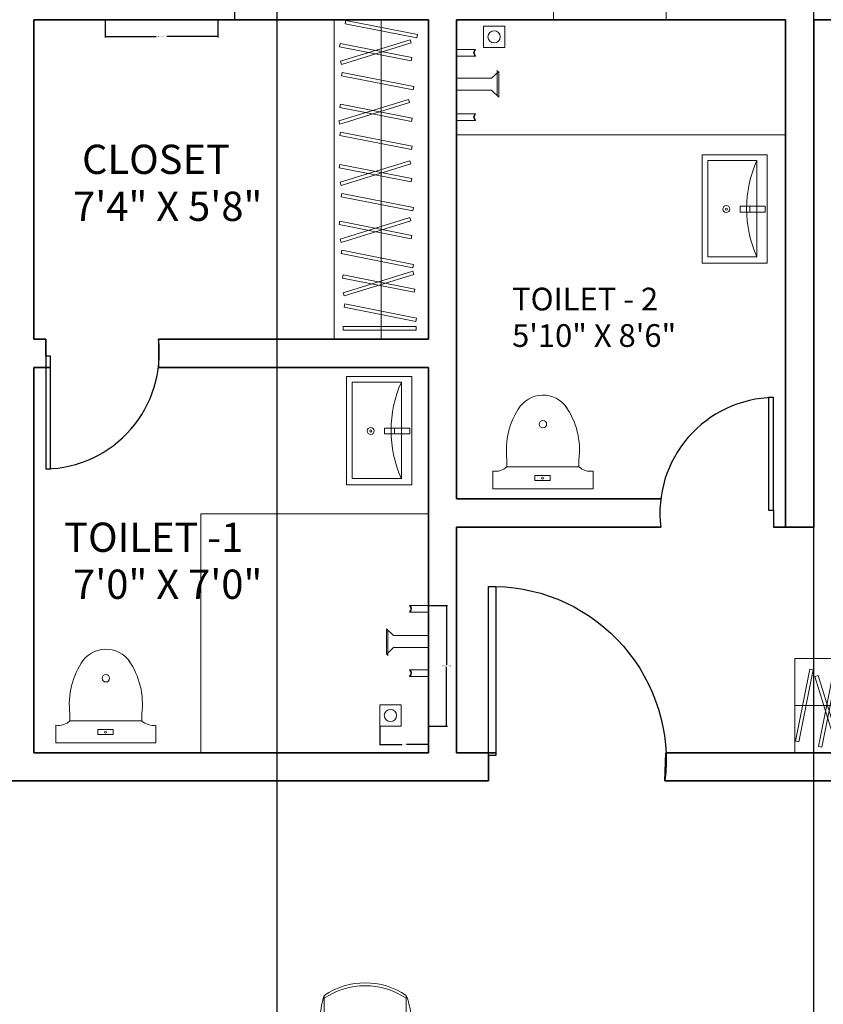
# Model space of a CAD drawing. Units: inches. Extents: x -61 to 1599, y -1316 to 257.
# Tile 202 of 204: x 1213 to 1384, y -61 to 149. Entities that reach past the tile are written whole.
import ezdxf

# ---------------------------------------------------------------- set-up
doc = ezdxf.new("R2010")
doc.units = ezdxf.units.IN
doc.header["$MEASUREMENT"] = 0
doc.linetypes.add('ACAD_ISO02W100', pattern=[15, 12, -3])
for name, color, linetype, lineweight in [('A-ANNO-DIMS', 2, 'Continuous', 18), ('A-AREA-IDEN', 1, 'Continuous', 18), ('A-FLOR-CASE', 8, 'Continuous', 18), ('A-FLOR-FIXT', 8, 'Continuous', 18), ('A-WALL-JAMB', 4, 'ACAD_ISO02W100', 25), ('DOORS', 2, 'Continuous', 25), ('FURNITURE', 83, 'Continuous', 18), ('WALLS', 4, 'Continuous', 35), ('WINDOWS', 220, 'Continuous', 18)]:
    doc.layers.add(name, color=color, linetype=linetype, lineweight=lineweight)
doc.styles.get("Standard").update_dxf_attribs({"font": 'arial.ttf'})
doc.dimstyles.get("Standard").update_dxf_attribs({"dimtxt": 0.18, "dimasz": 0.18, "dimexe": 0.18, "dimexo": 0.0625, "dimgap": 0.09, "dimtad": 0, "dimtih": 1, "dimtoh": 1, "dimdec": 0, "dimzin": 0, "dimdsep": 46, "dimlunit": 3, "dimtxsty": 'Standard', "dimcen": 0.09, "dimadec": 0, "dimazin": 0, "dimtfac": 1, "dimtdec": 0, "dimtofl": 0, "dimtmove": 0, "dimatfit": 3, "dimfxl": 1, "dimtolj": 1, "dimtzin": 0, "dimarcsym": 0})

# ---------------------------------------------------------------- blocks, each defined once
blk = doc.blocks.new('DOOR-SWING-24')
blk.add_line((0, 0), (0, 3.6))
blk.add_lwpolyline([(0, 0), (0, -24), (1.05, -24), (1.05, 0)], close=True)
blk.add_arc((-0.44, 0.62), 24.62, 271.0259, 6.9559)
blk = doc.blocks.new('DOOR-SWING-36')
blk.add_line((0, 0), (0, -5.4))
blk.add_lwpolyline([(0, 0), (0, 36), (-1.57, 36), (-1.57, 0)], close=True)
blk.add_arc((-0.74, -1.08), 37.09, 91.2913, 186.6905)
blk = doc.blocks.new('WIN-24IN')
for p, q in [((0, 4.5), (0, 9)), ((0, 9), (0, 0)), ((24, 9), (24, 0)), ((0, 5.19), (24, 5.19)), ((0, 4.5), (24, 4.5))]:
    blk.add_line(p, q)
blk = doc.blocks.new('WC-FLOOR-MOUNT')
for p, q in [((3.02, 4.69), (3.02, 6.17)), ((3.02, 4.69), (18.31, 4.69)), ((18.31, 4.69), (18.31, 6.17)), ((0, 0), (0, 3.75)), ((21.33, 0), (21.33, 3.75)), ((0, 0), (21.33, 0))]:
    blk.add_line(p, q)
blk.add_lwpolyline([(12.24, 1.73), (8.96, 1.73), (8.96, 2.81), (12.24, 2.81)], close=True)
for centre, radius in [((10.67, 13.73), 0.792), ((10.6, 2.27), 0.208)]:
    blk.add_circle(centre, radius)
for centre, radius, start, end in [((10.67, 13.73), 6.18, 27.6844, 141.4697), ((19.05, 8.26), 16.17, 144.824, 187.4232), ((2.28, 8.26), 16.17, 352.5768, 35.176), ((0.56, 7.25), 3.55, 260.8586, 313.6993), ((20.77, 7.25), 3.55, 226.3007, 279.1414)]:
    blk.add_arc(centre, radius, start, end)
blk = doc.blocks.new('LAVATORY-WALL')
blk.add_line((10.19, 12.11), (10.19, 10.88))
for points in [[(13.87, 0), (0, 0), (0, 23.07), (13.87, 23.07)], [(13.87, 0), (0, 0), (0, 23.07), (13.87, 23.07)], [(1.2, 1.34), (1.2, 21.88), (11.67, 21.88), (11.67, 1.34)], [(8.09, 10.88), (8.09, 12.11), (13.47, 12.11), (13.47, 10.88)]]:
    blk.add_lwpolyline(points, close=True)
for radius in [0.74, 0.233]:
    blk.add_circle((5.16, 11.5), radius)
blk.add_arc((34.73, 11.61), 25.25, 155.9939, 204.0061)
blk = doc.blocks.new('SHOWER-FITTINGS')
for p, q in [((10.35, 25.72), (6.31, 25.72)), ((10.35, 24.3), (6.31, 24.3)), ((10.35, 23), (10.35, 23)), ((2.92, 19.29), (1.4, 20.76)), ((1.4, 15.27), (1.4, 20.76)), ((1.69, 14.98), (1.69, 20.48)), ((10.35, 19.29), (2.92, 19.29)), ((2.92, 16.74), (1.4, 15.27)), ((10.35, 16.74), (2.92, 16.74)), ((10.35, 12.03), (6.31, 12.03)), ((10.35, 10.61), (6.31, 10.61))]:
    blk.add_line(p, q)
blk.add_lwpolyline([(4.52, 0), (0, 0), (0, 4.57), (4.52, 4.57)], close=True)
blk.add_circle((2.26, 2.29), 1.31)
for points in [[(6.31, 24.3), (6.45, 24.53), (6.75, 25), (6.46, 25.48), (6.31, 25.72)], [(6.45, 24.3), (6.59, 24.53), (6.88, 25), (6.59, 25.48), (6.45, 25.72)], [(6.31, 10.61), (6.45, 10.84), (6.75, 11.31), (6.46, 11.78), (6.31, 12.03)], [(6.45, 10.61), (6.59, 10.84), (6.88, 11.31), (6.59, 11.78), (6.45, 12.03)]]:
    blk.add_open_spline(points, degree=3, knots=[0, 0, 0, 0, 0.7501, 1.532449, 1.532449, 1.532449, 1.532449])
blk = doc.blocks.new('SHOWER-FITTINGS-2')
for p, q in [((0, 15.11), (4.04, 15.11)), ((0, 13.69), (4.04, 13.69)), ((8.66, 10.73), (8.66, 5.24)), ((0, 8.98), (7.43, 8.98)), ((7.43, 8.98), (8.95, 10.45)), ((8.95, 10.45), (8.95, 4.96)), ((0, 6.43), (7.43, 6.43)), ((7.43, 6.43), (8.95, 4.96)), ((0, 1.42), (4.04, 1.42)), ((0, 0), (4.04, 0))]:
    blk.add_line(p, q)
blk.add_lwpolyline([(10.23, 15.5), (5.71, 15.5), (5.71, 20.08), (10.23, 20.08)], close=True)
blk.add_circle((7.97, 17.79), 1.31)
for points in [[(3.91, 15.11), (3.76, 14.88), (3.47, 14.41), (3.76, 13.94), (3.91, 13.69)], [(4.04, 15.11), (3.9, 14.88), (3.6, 14.41), (3.89, 13.94), (4.04, 13.69)], [(3.91, 1.42), (3.76, 1.19), (3.47, 0.72), (3.76, 0.24), (3.91, 0)], [(4.04, 1.42), (3.9, 1.19), (3.6, 0.72), (3.89, 0.24), (4.04, 0)]]:
    blk.add_open_spline(points, degree=3, knots=[0, 0, 0, 0, 0.7501, 1.532449, 1.532449, 1.532449, 1.532449])
blk = doc.blocks.new('DINING-CHAIR')
for p, q in [((0.9, 2.16), (0.9, 13.35)), ((18.35, 2.16), (18.35, 13.35))]:
    blk.add_line(p, q)
for centre, radius, start, end in [((9.63, 0.52), 15.52, 55.8098, 124.1902), ((9.63, -0.1), 15.52, 55.8098, 124.1902), ((17.78, 7.76), 17.78, 161.6455, 198.3545), ((4.51, 7.76), 14.92, 337.9646, 22.0354), ((9.63, 12.87), 12.87, 227.332, 312.668)]:
    blk.add_arc(centre, radius, start, end)
blk = doc.blocks.new('WARDROBE-HANGING')
blk.add_line((10.05, 0), (10.05, 68))
for points in [[(20.09, 0), (0, 0), (0, 68), (20.09, 68)], [(2.48, 67.85), (17.75, 64.85), (17.61, 64.14), (2.34, 67.15)], [(1.32, 62.96), (16.59, 59.95), (16.45, 59.25), (1.19, 62.25)], [(1.35, 59.16), (16.22, 63.73), (16.43, 63.04), (1.56, 58.47)], [(1.71, 56.78), (16.98, 53.78), (16.84, 53.07), (1.57, 56.08)], [(1, 46.47), (15.87, 51.04), (16.08, 50.35), (1.21, 45.78)], [(1.39, 50.01), (16.66, 47.01), (16.52, 46.3), (1.26, 49.31)], [(1.36, 44.09), (16.63, 41.09), (16.49, 40.38), (1.23, 43.38)], [(1.28, 33.41), (16.16, 37.98), (16.37, 37.29), (1.49, 32.72)], [(1.26, 37.2), (16.53, 34.2), (16.39, 33.49), (1.12, 36.5)], [(1.65, 31.03), (16.92, 28.03), (16.78, 27.32), (1.51, 30.32)], [(1.28, 21.3), (16.15, 25.87), (16.36, 25.18), (1.49, 20.61)], [(1.26, 25.09), (16.53, 22.09), (16.39, 21.38), (1.12, 24.39)], [(1.65, 18.92), (16.91, 15.92), (16.78, 15.21), (1.51, 18.21)], [(1.91, 13.69), (17.17, 10.68), (17.04, 9.98), (1.77, 12.98)], [(1.93, 9.89), (16.8, 14.46), (17.01, 13.77), (2.14, 9.2)], [(2.29, 7.51), (17.56, 4.51), (17.42, 3.8), (2.16, 6.81)], [(17.49, 1.96), (1.93, 1.96), (1.93, 2.68), (17.49, 2.68)]]:
    blk.add_lwpolyline(points, close=True)
blk = doc.blocks.new('*D614')
at = {"layer": 'A-ANNO-DIMS', "color": 0, "lineweight": -2, "transparency": 16777216}
for p, q in [((1230.88, 148.61), (1230.88, 144.9)), ((1254.88, 148.61), (1254.88, 144.9)), ((1231.06, 145.08), (1241.76, 145.08)), ((1254.7, 145.08), (1244, 145.08))]:
    blk.add_line(p, q, dxfattribs=at)
at = {"layer": 'A-ANNO-DIMS', "color": 0, "transparency": 16777216}
for points in [[(1231.06, 145.11), (1231.06, 145.05), (1230.88, 145.08)], [(1254.7, 145.11), (1254.7, 145.05), (1254.88, 145.08)]]:
    blk.add_solid(points, dxfattribs=at)
at = {"layer": 'DEFPOINTS', "color": 0, "transparency": 16777216}
for p in [(1230.88, 148.68), (1254.88, 148.68), (1254.88, 145.08)]:
    blk.add_point(p, dxfattribs=at)
at = {"layer": 'A-ANNO-DIMS', "color": 0, "transparency": 16777216, "insert": (1242.88, 145.08), "char_height": 0.18, "attachment_point": 5}
blk.add_mtext('\\A1;WINDOW 24 TYP.', dxfattribs=at)
blk = doc.blocks.new('*D615')
at = {"layer": 'A-ANNO-DIMS', "color": 0, "lineweight": -2, "transparency": 16777216}
for p, q in [((1254.94, 157.68), (1258.66, 157.68)), ((1258.48, 157.5), (1258.48, 153.36)), ((1258.48, 148.86), (1258.48, 153)), ((1254.94, 148.68), (1258.66, 148.68))]:
    blk.add_line(p, q, dxfattribs=at)
at = {"layer": 'A-ANNO-DIMS', "color": 0, "transparency": 16777216}
for points in [[(1258.45, 157.5), (1258.51, 157.5), (1258.48, 157.68)], [(1258.45, 148.86), (1258.51, 148.86), (1258.48, 148.68)]]:
    blk.add_solid(points, dxfattribs=at)
at = {"layer": 'DEFPOINTS', "color": 0, "transparency": 16777216}
for p in [(1254.88, 157.68), (1258.48, 157.68), (1254.88, 148.68)]:
    blk.add_point(p, dxfattribs=at)
at = {"layer": 'A-ANNO-DIMS', "color": 0, "transparency": 16777216, "insert": (1258.48, 153.18), "char_height": 0.18, "attachment_point": 5}
blk.add_mtext('\\A1;9 TYP.', dxfattribs=at)
blk = doc.blocks.new('*D650')
at = {"layer": 'A-ANNO-DIMS', "color": 0, "lineweight": -2, "transparency": 16777216}
for p, q in [((1299.77, 24.03), (1303.74, 24.03)), ((1303.56, 23.85), (1303.56, 11.35)), ((1303.56, -1.51), (1303.56, 10.99)), ((1299.77, -1.69), (1303.74, -1.69))]:
    blk.add_line(p, q, dxfattribs=at)
at = {"layer": 'A-ANNO-DIMS', "color": 0, "transparency": 16777216}
for points in [[(1303.53, 23.85), (1303.59, 23.85), (1303.56, 24.03)], [(1303.53, -1.51), (1303.59, -1.51), (1303.56, -1.69)]]:
    blk.add_solid(points, dxfattribs=at)
at = {"layer": 'DEFPOINTS', "color": 0, "transparency": 16777216}
for p in [(1299.7, 24.03), (1303.56, 24.03), (1299.7, -1.69)]:
    blk.add_point(p, dxfattribs=at)
at = {"layer": 'A-ANNO-DIMS', "color": 0, "transparency": 16777216, "insert": (1303.56, 11.17), "char_height": 0.18, "attachment_point": 5}
blk.add_mtext('\\A1;SHOWER 26 TYP.', dxfattribs=at)
blk = doc.blocks.new('*D651')
at = {"layer": 'A-ANNO-DIMS', "color": 0, "lineweight": -2, "transparency": 16777216}
for p, q in [((1289.35, -1.75), (1289.35, -5.73)), ((1299.7, -1.75), (1299.7, -5.73)), ((1289.53, -5.55), (1294.01, -5.55)), ((1299.52, -5.55), (1295.05, -5.55))]:
    blk.add_line(p, q, dxfattribs=at)
at = {"layer": 'A-ANNO-DIMS', "color": 0, "transparency": 16777216}
for points in [[(1289.53, -5.52), (1289.53, -5.58), (1289.35, -5.55)], [(1299.52, -5.52), (1299.52, -5.58), (1299.7, -5.55)]]:
    blk.add_solid(points, dxfattribs=at)
at = {"layer": 'DEFPOINTS', "color": 0, "transparency": 16777216}
for p in [(1289.35, -1.69), (1299.7, -1.69), (1299.7, -5.55)]:
    blk.add_point(p, dxfattribs=at)
at = {"layer": 'A-ANNO-DIMS', "color": 0, "transparency": 16777216, "insert": (1294.53, -5.55), "char_height": 0.18, "attachment_point": 5}
blk.add_mtext('\\A1;10 TYP.', dxfattribs=at)
blk = doc.blocks.new('*D708')
at = {"layer": 'A-ANNO-DIMS', "color": 0, "lineweight": -2, "transparency": 16777216}
for p, q in [((1267.48, -588.11), (1267.48, 257.46)), ((1267.66, 257.28), (1324.14, 257.28)), ((1381.52, 257.28), (1325.05, 257.28)), ((1381.7, -588.11), (1381.7, 257.46))]:
    blk.add_line(p, q, dxfattribs=at)
at = {"layer": 'A-ANNO-DIMS', "color": 0, "transparency": 16777216}
for points in [[(1267.66, 257.31), (1267.66, 257.25), (1267.48, 257.28)], [(1381.52, 257.31), (1381.52, 257.25), (1381.7, 257.28)]]:
    blk.add_solid(points, dxfattribs=at)
at = {"layer": 'DEFPOINTS', "color": 0, "transparency": 16777216}
for p in [(1381.7, 257.28), (1267.48, -588.17), (1381.7, -588.17)]:
    blk.add_point(p, dxfattribs=at)
at = {"layer": 'A-ANNO-DIMS', "color": 0, "transparency": 16777216, "insert": (1324.59, 257.28), "char_height": 0.18, "attachment_point": 5}
blk.add_mtext('\\A1;114.22', dxfattribs=at)

msp = doc.modelspace()

# ---------------------------------------------------------------- linework, layer by layer
at = {"layer": 'A-FLOR-FIXT'}
for p, q in [((1305.7028, 124.2077), (1375.7028, 124.2077)), ((1299.7028, 43.5315), (1251.2827, 43.5315)), ((1251.2827, 43.5315), (1251.2827, -7.3229))]:
    msp.add_line(p, q, dxfattribs=at)
at = {"layer": 'A-WALL-JAMB'}
for p, q in [((1218.2351, 80.6771), (1218.2351, 74.6771)), ((1242.2351, 80.6771), (1242.2306, 74.6771)), ((1312.4752, -13.3229), (1312.4752, -7.3229)), ((1350.0502, -13.3229), (1350.2648, -7.3229))]:
    msp.add_line(p, q, dxfattribs=at)
at = {"layer": 'WALLS'}
for p, q in [((1215.7028, 148.6771), (1215.7028, 80.6771)), ((1215.7028, 148.6771), (1299.7028, 148.6771)), ((1299.7028, 148.6771), (1299.7028, 80.6771)), ((1305.7028, 148.6771), (1305.7028, 46.6771)), ((1305.7028, 148.6771), (1375.7028, 148.6771)), ((1375.7028, 148.6771), (1375.7028, 40.6771)), ((1381.7028, 148.6771), (1381.7028, 40.6771)), ((1381.7028, 148.6771), (1513.7028, 148.6771)), ((1215.7028, 80.6771), (1218.2351, 80.6771)), ((1242.2351, 80.6771), (1299.7028, 80.6771)), ((1215.7028, 74.6771), (1215.7028, -7.3229)), ((1215.7028, 74.6771), (1219.2851, 74.6771)), ((1242.2306, 74.6771), (1299.7028, 74.6771)), ((1299.7028, 74.6771), (1299.7028, -7.3229)), ((1305.7028, 46.6771), (1349.1506, 46.6771)), ((1305.7028, 40.6771), (1305.7028, -7.3229)), ((1305.7028, 40.6771), (1349.1461, 40.6771)), ((1373.1461, 40.6771), (1381.7028, 40.6771)), ((1215.7028, -7.3229), (1299.7028, -7.3229)), ((1305.7028, -7.3229), (1314.0502, -7.3229)), ((1350.2648, -7.3229), (1381.7028, -7.3229)), ((1375.7028, -7.3229), (1513.7028, -7.3229)), ((1201.0506, -13.3229), (1215.7028, -13.3229)), ((1215.7028, -13.3229), (1305.7028, -13.3229)), ((1299.7028, -13.3229), (1312.4752, -13.3229)), ((1350.0502, -13.3229), (1381.7028, -13.3229)), ((1375.7028, -13.3229), (1513.7028, -13.3229))]:
    msp.add_line(p, q, dxfattribs=at)

# ---------------------------------------------------------------- block references
at = {"layer": 'A-FLOR-CASE'}
msp.add_blockref('WARDROBE-HANGING', (1279.609, 80.677), dxfattribs=at)
at = {"layer": 'A-FLOR-CASE', "rotation": 90.00000000000033}
msp.add_blockref('WARDROBE-HANGING', (1445.7029, -7.3231), dxfattribs=at)
at = {"layer": 'A-FLOR-FIXT'}
for name, p in [('SHOWER-FITTINGS-2', (1305.703, 127.237)), ('LAVATORY-WALL', (1357.936, 96.864)), ('LAVATORY-WALL', (1282.2705, 49.6634)), ('WC-FLOOR-MOUNT', (1313.402, 48.864)), ('SHOWER-FITTINGS', (1289.351, -1.689)), ('WC-FLOOR-MOUNT', (1220.3826, -5.2012))]:
    msp.add_blockref(name, p, dxfattribs=at)
at = {"layer": 'DOORS'}
msp.add_blockref('DOOR-SWING-24', (1218.2351, 77.0771), dxfattribs=at)
at = {"layer": 'DOORS', "rotation": 180}
msp.add_blockref('DOOR-SWING-24', (1373.1461, 44.2771), dxfattribs=at)
at = {"layer": 'DOORS', "extrusion": (0, 0, -1), "zscale": -1}
msp.add_blockref('DOOR-SWING-36', (-1312.4752, -7.9229), dxfattribs=at)
at = {"layer": 'FURNITURE'}
msp.add_blockref('DINING-CHAIR', (1276.622, -72.324), dxfattribs=at)
at = {"layer": 'WINDOWS'}
msp.add_blockref('WIN-24IN', (1326.3196, 148.677), dxfattribs=at)

# ---------------------------------------------------------------- texts
at = {"layer": 'A-AREA-IDEN'}
for s, height, p in [('   CLOSET', 6.22364, (1220.2634, 115.8502)), ('  7\'4" X 5\'8"', 6.223643, (1220.2634, 105.8525)), ('TOILET - 2', 4.8321, (1317.5043, 86.8095)), ('5\'10" X 8\'6"', 4.832098, (1317.5043, 79.0472)), (' TOILET -1', 6.22364, (1220.2634, 35.4228)), ('  7\'0" X 7\'0"', 6.223643, (1220.2634, 25.425))]:
    msp.add_text(s, height=height, dxfattribs=at).set_placement(p)

# ---------------------------------------------------------------- dimensions: what is measured, and where the dimension line sits
at = {"layer": 'A-ANNO-DIMS'}
dim = msp.add_linear_dim(base=(1381.7028, 257.2771), p1=(1267.4807, -588.169), p2=(1381.7028, -588.169), dimstyle='Standard', override={"dimdec": 2, "dimlfac": 1, "dimrnd": 0, "dimzin": 0, "dimdsep": 46, "dimlunit": 2}, dxfattribs=at)
dim.commit()
dim.dimension.update_dxf_attribs({"geometry": '*D708', "text_midpoint": (1324.5917, 257.2771)})
for base, p1, p2, text, picture, middle in [((1258.4825, 157.6771), (1254.8825, 148.6771), (1254.8825, 157.6771), '<> TYP.', '*D615', (1258.4825, 153.1771)), ((1303.5606, 24.03), (1299.7028, -1.6889), (1299.7028, 24.03), 'SHOWER <> TYP.', '*D650', (1303.5606, 11.1706))]:
    dim = msp.add_linear_dim(base=base, p1=p1, p2=p2, angle=90, text=text, dimstyle='Standard', override={"dimdec": 0, "dimlfac": 1, "dimrnd": 0, "dimzin": 0, "dimdsep": 46, "dimlunit": 2}, dxfattribs=at)
    dim.commit()
    dim.dimension.update_dxf_attribs({"geometry": picture, "text_midpoint": middle})
for base, p1, p2, text, picture, middle in [((1254.8825, 145.0771), (1230.8825, 148.6771), (1254.8825, 148.6771), 'WINDOW <> TYP.', '*D614', (1242.8825, 145.0771)), ((1299.7028, -5.5467), (1289.3512, -1.6889), (1299.7028, -1.6889), '<> TYP.', '*D651', (1294.527, -5.5467))]:
    dim = msp.add_linear_dim(base=base, p1=p1, p2=p2, text=text, dimstyle='Standard', override={"dimdec": 0, "dimlfac": 1, "dimrnd": 0, "dimzin": 0, "dimdsep": 46, "dimlunit": 2}, dxfattribs=at)
    dim.commit()
    dim.dimension.update_dxf_attribs({"geometry": picture, "text_midpoint": middle})

doc.saveas('drawing.dxf')
